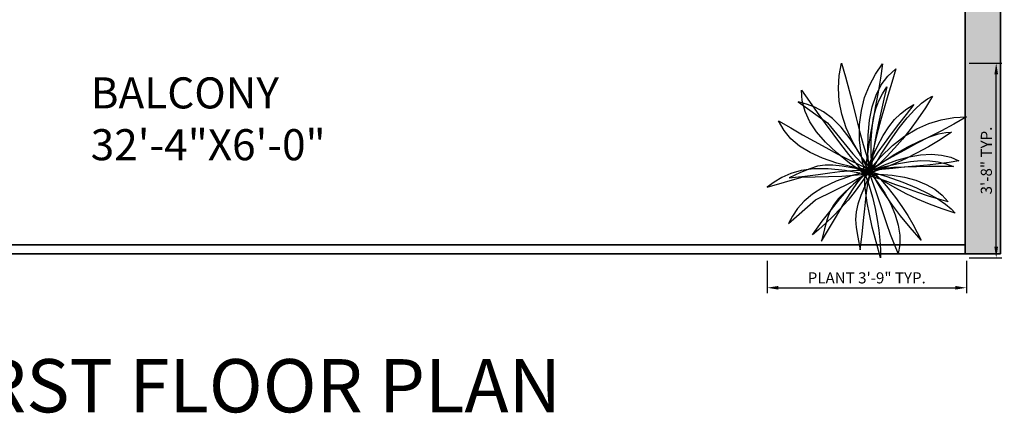
# Model space of a CAD drawing. Units: inches. Extents: x 1566 to 2546, y 1087 to 2705.
# Tile 13 of 27: x 2237 to 2459, y 1100 to 1189. Entities that reach past the tile are written whole.
import ezdxf

# ---------------------------------------------------------------- set-up
doc = ezdxf.new("R2010")
doc.units = ezdxf.units.IN
for name, color, linetype, lineweight in [('A-ANNO-DIMS', 2, 'Continuous', 18), ('A-AREA-IDEN', 7, 'Continuous', 18), ('A-WALL', 7, 'Continuous', 35), ('A-WALL-PATT', 8, 'Continuous', 13), ('L-PLNT', 94, 'Continuous', 18)]:
    doc.layers.add(name, color=color, linetype=linetype, lineweight=lineweight)
doc.layers.add('DIENHOA', color=3, linetype='Continuous')
doc.styles.get("Standard").update_dxf_attribs({"font": 'arial.ttf'})
doc.dimstyles.new('ISO-25', dxfattribs={"dimtxt": 2.5, "dimasz": 2.5, "dimexe": 1.25, "dimexo": 0.625, "dimtad": 1, "dimtxsty": 'Standard', "dimcen": 2.5, "dimadec": 0, "dimazin": 0, "dimtfac": 1, "dimtmove": 0, "dimatfit": 3, "dimfxl": 1, "dimarcsym": 0})

# ---------------------------------------------------------------- blocks, each defined once
blk = doc.blocks.new('Cay03_mb')
at = {"layer": 'DIENHOA'}
for p, q in [((118.6, 555.3), (166.2, 599.1)), ((166.2, 599.1), (142.2, 519.4)), ((79.5, 503.7), (118.6, 555.3)), ((48.6, 443.6), (79.5, 503.7)), ((142.2, 519.4), (119, 441.7)), ((25.5, 374.3), (48.6, 443.6)), ((119, 441.7), (96.7, 365.6)), ((-365.2, 390.3), (-414.4, 402.8)), ((-414.4, 402.8), (-240.2, 277.8)), ((-314.9, 371.3), (-365.2, 390.3)), ((-263.5, 343.5), (-314.9, 371.3)), ((9.9, 295.3), (25.5, 374.3)), ((96.7, 365.6), (75.6, 290.6)), ((-211.2, 304.6), (-263.5, 343.5)), ((-158, 252.3), (-211.2, 304.6)), ((1.6, 205.7), (9.9, 295.3)), ((363.4, 275.4), (436.8, 297.2)), ((436.8, 297.2), (511, 309.6)), ((511, 309.6), (585.9, 313.5)), ((585.9, 313.5), (511.8, 271.4)), ((-240.2, 277.8), (-88.4, 94.9)), ((-104.2, 184.4), (-158, 252.3)), ((75.6, 290.6), (55.7, 216.3)), ((218.5, 199.8), (290.6, 243.2)), ((290.6, 243.2), (363.4, 275.4)), ((511.8, 271.4), (437.6, 231.5)), ((-49.6, 98.5), (-104.2, 184.4)), ((0.2, 104.9), (1.6, 205.7)), ((55.7, 216.3), (37.3, 142.1)), ((147, 144.1), (218.5, 199.8)), ((363.7, 192.9), (290.2, 154.9)), ((437.6, 231.5), (363.7, 192.9)), ((37.3, 142.1), (20.5, 67.6)), ((75.9, 75.2), (147, 144.1)), ((290.2, 154.9), (217.4, 116.6)), ((-88.4, 94.9), (5.4, -7.8)), ((5.4, -7.8), (-49.6, 98.5)), ((5.4, -7.8), (0.2, 104.9)), ((5.4, -7.8), (75.9, 75.2)), ((20.5, 67.6), (5.4, -7.8)), ((145.5, 77.3), (74.7, 36.1)), ((217.4, 116.6), (145.5, 77.3)), ((-345, 5.4), (-399.6, -17.1)), ((-298.6, 20.1), (-345, 5.4)), ((-254.7, 27.4), (-298.6, 20.1)), ((-208, 27.8), (-254.7, 27.4)), ((-152.7, 21.7), (-208, 27.8)), ((-83.4, 9.7), (-152.7, 21.7)), ((5.4, -7.8), (-83.4, 9.7)), ((74.7, 36.1), (5.4, -7.8)), ((5.4, -7.8), (100.3, 18.4)), ((46.3, 0.9), (5.4, -7.8)), ((96.7, 7.5), (46.3, 0.9)), ((155, 12.2), (96.7, 7.5)), ((100.3, 18.4), (182.2, 37.2)), ((219.6, 15.4), (155, 12.2)), ((182.2, 37.2), (253, 48.9)), ((289, 17.4), (219.6, 15.4)), ((253, 48.9), (314.6, 54.1)), ((361.6, 18.5), (289, 17.4)), ((314.6, 54.1), (369.2, 53.3)), ((435.8, 18.9), (361.6, 18.5)), ((369.2, 53.3), (418.6, 46.8)), ((418.6, 46.8), (464.9, 35.2)), ((510, 19), (435.8, 18.9)), ((464.9, 35.2), (510, 19)), ((-399.6, -17.1), (-468, -47.9)), ((-468, -47.9), (-375.6, -37.8)), ((-375.6, -37.8), (-295.3, -27.9)), ((-295.3, -27.9), (-225.8, -18.9)), ((-225.8, -18.9), (-165.8, -11.3)), ((-165.8, -11.3), (-114, -5.7)), ((-114, -5.7), (-69, -2.9)), ((-79.8, -79.6), (-45.1, -46.3)), ((-69, -2.9), (-29.6, -3.4)), ((-45.1, -46.3), (-16.5, -22.4)), ((5.4, -7.8), (-33.2, -69.5)), ((-29.6, -3.4), (5.4, -7.8)), ((-16.5, -22.4), (5.4, -7.8)), ((5.4, -7.8), (56.8, -73.3)), ((25.9, -64.4), (5.4, -7.8)), ((5.4, -7.8), (112.8, -40.3)), ((53.5, -41.6), (5.4, -7.8)), ((107, -75.7), (53.5, -41.6)), ((112.8, -40.3), (207.5, -73.8)), ((-120.2, -122.1), (-79.8, -79.6)), ((-33.2, -69.5), (-74.6, -127.3)), ((47, -125.9), (25.9, -64.4)), ((56.8, -73.3), (100.4, -139.1)), ((165.5, -109.6), (107, -75.7)), ((228.7, -142.8), (165.5, -109.6)), ((207.5, -73.8), (289.5, -107.6)), ((289.5, -107.6), (359.3, -141.1)), ((-216.3, -235.6), (-165.9, -174.1)), ((-165.9, -174.1), (-120.2, -122.1)), ((-74.6, -127.3), (-117.8, -181.1)), ((68.7, -190.6), (47, -125.9)), ((100.4, -139.1), (135.9, -204.3)), ((296, -174.7), (228.7, -142.8)), ((367.1, -204.8), (296, -174.7)), ((359.3, -141.1), (416.9, -173.5)), ((416.9, -173.5), (462.6, -204.2)), ((-162.1, -230.9), (-206.3, -276.5)), ((-117.8, -181.1), (-162.1, -230.9)), ((90.8, -256.6), (68.7, -190.6)), ((135.9, -204.3), (162.8, -268.3)), ((441.6, -232.7), (367.1, -204.8)), ((518.9, -257.7), (441.6, -232.7)), ((462.6, -204.2), (496.5, -232.5)), ((496.5, -232.5), (518.9, -257.7)), ((-271, -306.6), (-216.3, -235.6)), ((-206.3, -276.5), (-249.6, -317.8)), ((113.1, -322.2), (90.8, -256.6)), ((162.8, -268.3), (181, -330.4)), ((-329.5, -387.1), (-271, -306.6)), ((-249.6, -317.8), (-291, -354.7)), ((135.4, -385.6), (113.1, -322.2)), ((181, -330.4), (190, -390)), ((-291, -354.7), (-329.5, -387.1)), ((157.6, -445), (135.4, -385.6)), ((190, -390), (189.6, -446.3)), ((179.5, -498.7), (157.6, -445)), ((189.6, -446.3), (179.5, -498.7))]:
    blk.add_line(p, q, dxfattribs=at)
for points in [[(23.7, -5.4), (-41, 82.2), (-91.8, 167.1), (-129.7, 249.5), (-155.6, 329.6), (-170.2, 407.8), (-174.7, 484.2), (-169.8, 559.3), (-156.5, 633.1)], [(-156.5, 633.1), (-132.5, 551.3), (-110.5, 470), (-89.8, 389.2), (-69.6, 309), (-49, 229.4), (-27.1, 150.4), (-3.2, 72.1), (23.7, -5.4)], [(-16.4, -26.7), (-38.3, 80), (-48.9, 178.3), (-48.7, 269), (-38.5, 352.6), (-19.1, 429.7), (9, 501), (44.9, 567.1), (87.9, 628.5)], [(87.9, 628.5), (75.5, 544.2), (61.3, 461.2), (46.1, 379.1), (30.8, 297.8), (16.1, 216.9), (2.9, 136), (-8.3, 54.9), (-16.4, -26.7)], [(-395.6, 473.7), (-347.5, 405.6), (-300.6, 339.5), (-254.3, 275.1), (-208.3, 212.3), (-161.9, 150.9), (-114.8, 90.7), (-66.5, 31.6), (-16.4, -26.7)], [(-16.4, -26.7), (-108.3, 38.6), (-186.9, 101.7), (-252.4, 163.5), (-305.1, 224.4), (-345.4, 285.2), (-373.7, 346.6), (-390.4, 409.2), (-395.6, 473.7)], [(23.7, -5.4), (19.8, 93), (20.3, 177), (25, 248.5), (34, 309.8), (47.3, 362.7), (64.9, 409.3), (86.8, 451.7), (112.9, 491.9)], [(112.9, 491.9), (96, 419.7), (79.5, 347.4), (63.9, 276.5), (50, 208.4), (38.4, 144.8), (29.7, 86.9), (24.6, 36.3), (23.7, -5.4)], [(384.3, 437.5), (342.2, 367.8), (298.1, 301.7), (252.6, 239.4), (206.1, 181.1), (159.4, 127.2), (113, 78), (67.6, 33.6), (23.7, -5.4)], [(23.7, -5.4), (79.9, 91.7), (134.1, 176.2), (185.8, 248.4), (234.3, 308.7), (279, 357.3), (319.3, 394.8), (354.6, 421.4), (384.3, 437.5)], [(273.2, 387.3), (227.6, 328.8), (182.3, 270.1), (138.4, 212.3), (97.2, 156.4), (60, 103.4), (27.8, 54.6), (1.9, 10.8), (-16.4, -26.7)], [(-16.4, -26.7), (21.4, 64.2), (57, 140.3), (91.4, 203.3), (125.2, 255.1), (159.5, 297.5), (195, 332.5), (232.7, 361.8), (273.2, 387.3)], [(-530.5, 289.7), (-458.3, 248.1), (-387.9, 207.8), (-318.9, 168.7), (-250.8, 131.1), (-182.9, 94.8), (-114.9, 59.9), (-46.2, 26.5), (23.7, -5.4)], [(23.7, -5.4), (-87.2, 15.2), (-185, 39.6), (-270.3, 68.2), (-343.7, 101.4), (-405.9, 139.7), (-457.3, 183.5), (-498.7, 233.4), (-530.5, 289.7)], [(496.7, 224), (429.4, 178.4), (361.6, 136.9), (294.1, 99.5), (227.5, 66.1), (162.4, 36.7), (99.7, 11.5), (39.8, -9.7), (-16.4, -26.7)], [(-16.4, -26.7), (75.4, 37.9), (160.1, 91.8), (237.3, 135.7), (306.6, 170), (367.6, 195.4), (419.9, 212.5), (463.1, 221.9), (496.7, 224)], [(23.7, -5.4), (99.3, 29.7), (173.2, 57.1), (244.8, 76.7), (313.3, 88.3), (377.9, 91.8), (437.9, 87), (492.7, 73.8), (541.4, 52)], [(-16.4, -26.7), (-134, -4.7), (-235.3, 5.3), (-322, 4.7), (-395.9, -5), (-458.7, -22.3), (-512.3, -45.7), (-558.2, -73.6), (-598.4, -104.7)], [(541.4, 52), (484.1, 42.9), (421.2, 34.8), (354.4, 27.6), (285.4, 20.9), (216.1, 14.5), (148.2, 8.1), (83.5, 1.6), (23.7, -5.4)], [(-598.4, -104.7), (-392.7, -44.4), (-155, -37.4), (-16.4, -26.7)], [(-471.9, -320.3), (-310.5, -179.3), (-97.7, -73.3), (23.7, -5.4)], [(23.7, -5.4), (-92.3, -34.8), (-188.4, -68.2), (-266.9, -105.1), (-329.9, -144.9), (-379.7, -187), (-418.5, -230.7), (-448.5, -275.3), (-471.9, -320.3)], [(-276.2, -424.4), (-227.3, -345.4), (-185.7, -276.1), (-150, -215.7), (-119.1, -163.8), (-91.5, -119.5), (-66, -82.3), (-41.4, -51.6), (-16.4, -26.7)], [(-16.4, -26.7), (-84.9, -86), (-137, -133.1), (-175.8, -173), (-204.3, -210), (-225.5, -249.1), (-242.5, -294.7), (-258.4, -351.6), (-276.2, -424.4)], [(23.7, -5.4), (-13.6, -87.9), (-41.1, -152.6), (-59.6, -205), (-69.9, -250.7), (-72.8, -295), (-69.2, -343.6), (-59.7, -401.9), (-45.3, -475.5)], [(-45.3, -475.5), (-34.1, -383.2), (-25.4, -302.8), (-18.3, -233.1), (-12, -172.9), (-5.6, -121.2), (2, -76.8), (11.4, -38.5), (23.7, -5.4)], [(76.2, -524.2), (48.8, -428.5), (26.6, -341.7), (9.2, -264.1), (-3.6, -196.1), (-12.3, -138), (-17.1, -90.2), (-18.3, -53), (-16.4, -26.7)], [(-16.4, -26.7), (66.9, -26.6), (145.6, -32.7), (218.8, -44.9), (285.8, -63.1), (345.9, -87.1), (398.4, -116.6), (442.6, -151.6), (477.6, -191.8)], [(477.6, -191.8), (421.8, -176), (361.3, -156.9), (297.6, -135.5), (232.2, -112.6), (166.6, -89.4), (102.3, -66.6), (40.8, -45.4), (-16.4, -26.7)], [(-16.4, -26.7), (8.5, -95.1), (28.5, -163.3), (44.3, -230.6), (56.3, -296.1), (65, -359), (70.9, -418.5), (74.5, -473.9), (76.2, -524.2)], [(316.5, -418.1), (251.4, -342.8), (194.8, -273.3), (146.5, -210.2), (106.3, -153.8), (74.1, -104.7), (49.7, -63.4), (32.9, -30.1), (23.7, -5.4)], [(23.7, -5.4), (74.9, -57.1), (121.8, -110.6), (164.3, -165), (202.7, -219.4), (237, -272.9), (267.3, -324.5), (293.7, -373.2), (316.5, -418.1)]]:
    blk.add_lwpolyline(points, dxfattribs=at)
blk = doc.blocks.new('*D43')
at = {"layer": 'A-ANNO-DIMS', "color": 0, "lineweight": -2, "transparency": 16777216}
for p, q in [((2405.71, 1134.88), (2405.71, 1127.53)), ((2450.59, 1134.88), (2450.59, 1127.53)), ((2408.21, 1128.78), (2448.09, 1128.78))]:
    blk.add_line(p, q, dxfattribs=at)
at = {"layer": 'A-ANNO-DIMS', "color": 0, "transparency": 16777216}
for points in [[(2408.21, 1129.19), (2408.21, 1128.36), (2405.71, 1128.78)], [(2448.09, 1129.19), (2448.09, 1128.36), (2450.59, 1128.78)]]:
    blk.add_solid(points, dxfattribs=at)
at = {"layer": 'Defpoints', "color": 0, "transparency": 16777216}
for p in [(2405.71, 1135.51), (2450.59, 1135.51), (2450.59, 1128.78)]:
    blk.add_point(p, dxfattribs=at)
at = {"layer": 'A-ANNO-DIMS', "color": 0, "transparency": 16777216, "insert": (2428.15, 1130.68), "char_height": 2.5, "attachment_point": 5}
blk.add_mtext('PLANT 3\'-9" TYP.', dxfattribs=at)
blk = doc.blocks.new('*D44')
at = {"layer": 'A-ANNO-DIMS', "color": 0, "lineweight": -2, "transparency": 16777216}
for p, q in [((2451.22, 1179.36), (2458.57, 1179.36)), ((2457.32, 1138.01), (2457.32, 1176.86)), ((2451.22, 1135.51), (2458.57, 1135.51))]:
    blk.add_line(p, q, dxfattribs=at)
at = {"layer": 'A-ANNO-DIMS', "color": 0, "transparency": 16777216}
for points in [[(2456.91, 1176.86), (2457.74, 1176.86), (2457.32, 1179.36)], [(2456.91, 1138.01), (2457.74, 1138.01), (2457.32, 1135.51)]]:
    blk.add_solid(points, dxfattribs=at)
at = {"layer": 'Defpoints', "color": 0, "transparency": 16777216}
for p in [(2450.59, 1179.36), (2457.32, 1179.36), (2450.59, 1135.51)]:
    blk.add_point(p, dxfattribs=at)
at = {"layer": 'A-ANNO-DIMS', "color": 0, "transparency": 16777216, "insert": (2455.42, 1157.44), "char_height": 2.5, "attachment_point": 5, "rotation": 90}
blk.add_mtext('3\'-8" TYP.', dxfattribs=at)

msp = doc.modelspace()

# ---------------------------------------------------------------- hatches: boundary and pattern name
at = {"layer": 'A-WALL-PATT'}
h = msp.add_hatch(color=256, dxfattribs=at)
h.dxf.hatch_style = 1
h.paths.add_polyline_path([(2106.29, 1385.43), (2228.29, 1385.43), (2228.29, 1391.43), (2224.29, 1391.43), (2224.29, 1389.43), (2106.29, 1389.43), (2106.29, 1402.93), (2098.29, 1402.93), (2098.29, 1343.43), (2106.29, 1343.43), (2106.29, 1347.74)], flags=17)
h.paths.add_polyline_path([(2106.29, 1259.43), (2098.29, 1259.43), (2098.29, 1209.43), (2155.29, 1209.43), (2155.29, 1217.43), (2143.41, 1217.43), (2106.29, 1217.43)], flags=17)
h.paths.add_polyline_path([(2334.29, 1217.43), (2280.29, 1217.43), (2280.29, 1389.43), (2284.29, 1389.43), (2284.29, 1391.43), (2284.29, 1393.43), (2276.29, 1393.43), (2276.29, 1217.43), (2227.29, 1217.43), (2227.29, 1209.43), (2334.29, 1209.43)], flags=17)
h.paths.add_polyline_path([(2106.29, 1486.43), (2098.29, 1486.43), (2098.29, 1460.88), (2099.11, 1461.64), (2100.44, 1462.65), (2101.57, 1463.26), (2099.97, 1460.62), (2098.29, 1458.1), (2098.29, 1456.93), (2100.35, 1456.93), (2100.77, 1457.12), (2103.56, 1457.95), (2106.29, 1458.4), (2106.29, 1470.43), (2224.29, 1470.43), (2224.29, 1427.43), (2228.29, 1427.43), (2228.29, 1474.43), (2192.29, 1474.43), (2192.29, 1476.43), (2188.29, 1476.43), (2188.29, 1474.43), (2106.29, 1474.43)], flags=17)
h.paths.add_polyline_path([(2106.29, 1585.43), (2192.29, 1585.43), (2192.29, 1589.43), (2098.29, 1589.43), (2098.29, 1573.93), (2106.29, 1573.93)], flags=17)
h.paths.add_polyline_path([(2228.29, 1585.43), (2232.29, 1585.43), (2232.29, 1589.43), (2224.29, 1589.43), (2222.29, 1589.43), (2222.29, 1585.43), (2224.29, 1585.43), (2224.29, 1532.43), (2106.29, 1532.43), (2106.29, 1543.93), (2098.29, 1543.93), (2098.29, 1516.43), (2106.29, 1516.43), (2106.29, 1528.43), (2188.29, 1528.43), (2188.29, 1506.43), (2192.29, 1506.43), (2192.29, 1528.43), (2224.29, 1528.43), (2224.29, 1506.43), (2228.29, 1506.43)], flags=17)
h.paths.add_polyline_path([(2106.29, 1680.43), (2098.29, 1680.43), (2098.29, 1625.43), (2106.29, 1625.43)], flags=17)
h.paths.add_polyline_path([(2458.29, 1784.43), (2098.29, 1784.43), (2098.29, 1776.43), (2276.29, 1776.43), (2276.29, 1589.43), (2268.29, 1589.43), (2268.29, 1585.43), (2280.29, 1585.43), (2280.29, 1652.43), (2284.29, 1652.43), (2284.29, 1656.43), (2280.29, 1656.43), (2280.29, 1776.43), (2398.29, 1776.43), (2398.29, 1746.43), (2402.29, 1746.43), (2402.29, 1776.43), (2450.29, 1776.43), (2450.29, 1532.43), (2375.49, 1532.43), (2328.29, 1532.43), (2328.29, 1612.43), (2324.29, 1612.43), (2324.29, 1528.43), (2450.29, 1528.43), (2450.29, 1447.43), (2291.29, 1447.43), (2291.29, 1443.43), (2324.29, 1443.43), (2324.29, 1393.43), (2320.29, 1393.43), (2320.29, 1389.43), (2330.29, 1389.43), (2330.29, 1393.43), (2328.29, 1393.43), (2328.29, 1443.43), (2412.29, 1443.43), (2412.29, 1433.43), (2416.29, 1433.43), (2416.29, 1443.43), (2450.29, 1443.43), (2450.29, 1393.43), (2416.29, 1393.43), (2416.29, 1403.43), (2412.29, 1403.43), (2412.29, 1393.43), (2360.29, 1393.43), (2360.29, 1389.43), (2450.29, 1389.43), (2450.29, 1217.43), (2396.29, 1217.43), (2396.29, 1209.43), (2450.29, 1209.43), (2450.29, 1136.43), (2458.29, 1136.43)])

# ---------------------------------------------------------------- linework, layer by layer
at = {"layer": 'A-WALL'}
for p, q in [((2458.29, 1784.43), (2458.29, 1136.43)), ((2450.29, 1209.43), (2450.29, 1136.43)), ((2062.29, 1136.43), (2458.29, 1136.43)), ((2064.29, 1138.43), (2450.29, 1138.43))]:
    msp.add_line(p, q, dxfattribs=at)

# ---------------------------------------------------------------- block references
at = {"layer": 'L-PLNT', "xscale": 0.0378941924884598, "yscale": 0.0378941924884598, "zscale": 0.0378941924884598}
msp.add_blockref('Cay03_mb', (2428.39, 1155.37), dxfattribs=at)

# ---------------------------------------------------------------- texts
at = {"layer": 'A-AREA-IDEN', "attachment_point": 1}
for s, width, insert, char_height in [('BALCONY\\P32\'-4"X6\'-0"', 111.7553, (2253.22, 1176.17), 7), ('FIRST FLOOR PLAN', 179.2212, (2214.47, 1112.71), 12)]:
    msp.add_mtext_dynamic_manual_height_columns(s, width=width, gutter_width=12.5, heights=[0], dxfattribs=dict(at, insert=insert, char_height=char_height))

# ---------------------------------------------------------------- dimensions: what is measured, and where the dimension line sits
at = {"layer": 'A-ANNO-DIMS'}
dim = msp.add_linear_dim(base=(2457.3223, 1179.3647), p1=(2450.5907, 1135.5088), p2=(2450.5907, 1179.3647), angle=90, text='<> TYP.', dimstyle='ISO-25', override={"dimdec": 1, "dimrnd": 0, "dimzin": 1, "dimlunit": 4, "dimfrac": 2}, dxfattribs=at)
dim.commit()
dim.dimension.update_dxf_attribs({"geometry": '*D44', "text_midpoint": (2455.42, 1157.4367)})
dim = msp.add_linear_dim(base=(2450.59, 1128.78), p1=(2405.71, 1135.51), p2=(2450.59, 1135.51), text='PLANT <> TYP.', dimstyle='ISO-25', override={"dimdec": 1, "dimrnd": 0, "dimzin": 1, "dimlunit": 4, "dimfrac": 2}, dxfattribs=at)
dim.commit()
dim.dimension.update_dxf_attribs({"geometry": '*D43', "text_midpoint": (2428.15, 1130.68)})

doc.saveas('drawing.dxf')
